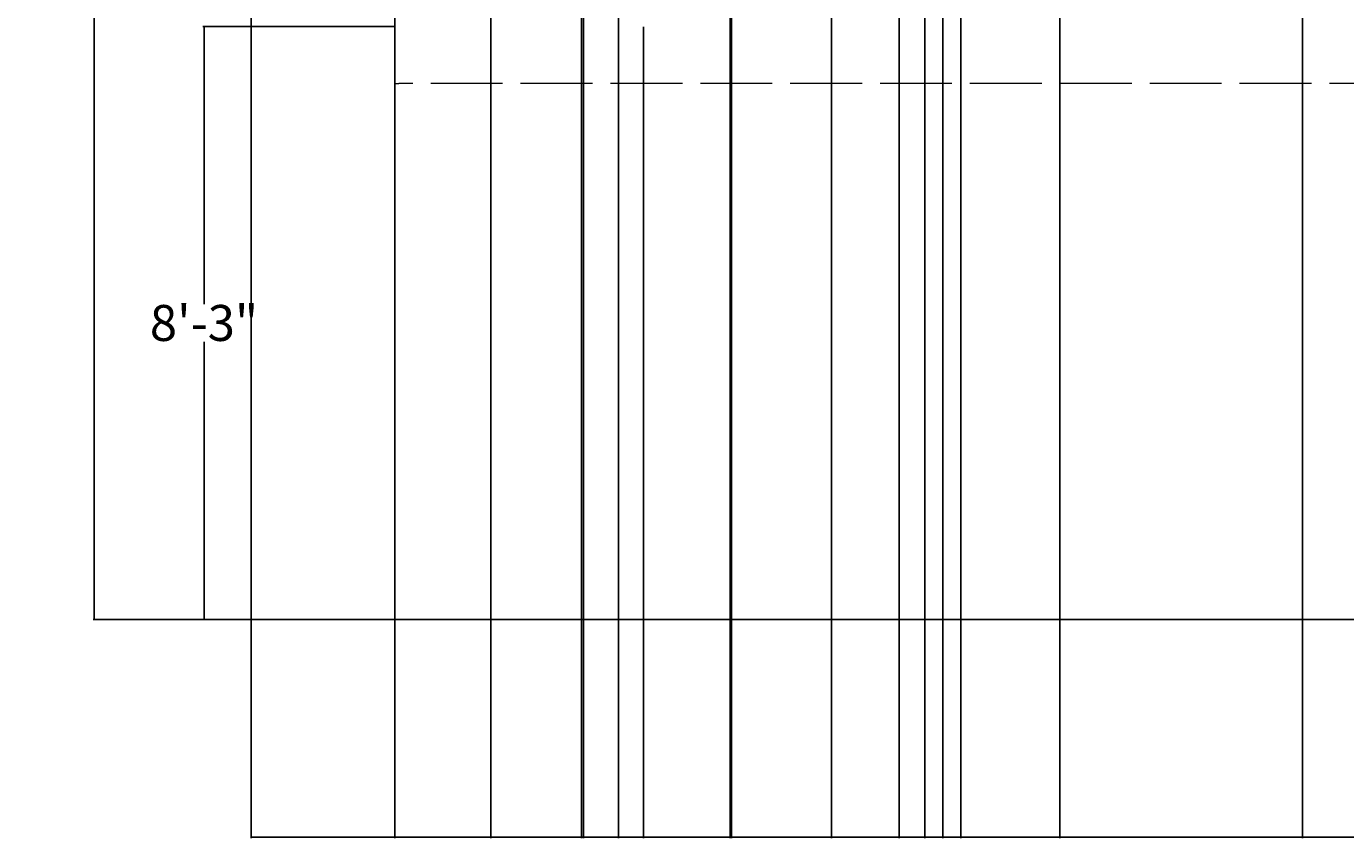
# Model space of a CAD drawing. Units: inches. Extents: x -36 to 401, y -686 to 73.
# Tile 1 of 15: x -36 to 184, y -686 to -550. Entities that reach past the tile are written whole.
import ezdxf

# ---------------------------------------------------------------- set-up
doc = ezdxf.new("R2010")
doc.units = ezdxf.units.IN
doc.header["$MEASUREMENT"] = 0
doc.linetypes.add('ACAD_ISO02W100', pattern=[15, 12, -3])
for name, color, linetype, lineweight in [('A-ANNO-DIMS', 2, 'Continuous', 18), ('A-FLOR-OVHD', 8, 'ACAD_ISO02W100', 18), ('C-PROP', 7, 'Continuous', 25)]:
    doc.layers.add(name, color=color, linetype=linetype, lineweight=lineweight)
doc.styles.get("Standard").update_dxf_attribs({"font": 'arial.ttf'})
doc.dimstyles.get("Standard").update_dxf_attribs({"dimtxt": 0.18, "dimasz": 0.18, "dimexe": 0.18, "dimexo": 0.0625, "dimgap": 0.09, "dimtad": 0, "dimtih": 1, "dimtoh": 1, "dimdec": 0, "dimzin": 0, "dimdsep": 46, "dimlunit": 3, "dimtxsty": 'Standard', "dimcen": 0.09, "dimadec": 0, "dimazin": 0, "dimtfac": 1, "dimtdec": 0, "dimtofl": 0, "dimtmove": 0, "dimatfit": 3, "dimfxl": 1, "dimtolj": 1, "dimtzin": 0, "dimarcsym": 0})

# ---------------------------------------------------------------- blocks, each defined once
blk = doc.blocks.new('*D8')
at = {"layer": 'A-ANNO-DIMS', "color": 0, "lineweight": -2, "transparency": 16777216}
for p, q in [((25.63, 7.79), (-24.68, 7.79)), ((-24.5, 7.61), (-24.5, -317.56)), ((-24.5, -649.03), (-24.5, -323.86)), ((1.63, -649.21), (-24.68, -649.21))]:
    blk.add_line(p, q, dxfattribs=at)
at = {"layer": 'A-ANNO-DIMS', "color": 0, "transparency": 16777216}
for points in [[(-24.53, 7.61), (-24.47, 7.61), (-24.5, 7.79)], [(-24.53, -649.03), (-24.47, -649.03), (-24.5, -649.21)]]:
    blk.add_solid(points, dxfattribs=at)
at = {"layer": 'Defpoints', "color": 0, "transparency": 16777216}
for p in [(25.69, 7.79), (-24.5, -649.21), (1.69, -649.21)]:
    blk.add_point(p, dxfattribs=at)
at = {"layer": 'A-ANNO-DIMS', "color": 0, "transparency": 16777216, "insert": (-24.5, -320.71), "char_height": 6, "attachment_point": 5}
blk.add_mtext('\\A1;54\'-9"', dxfattribs=at)
blk = doc.blocks.new('*D12')
at = {"layer": 'A-ANNO-DIMS', "color": 0, "lineweight": -2, "transparency": 16777216}
for p, q in [((25.63, -550.21), (-6.34, -550.21)), ((-6.16, -550.39), (-6.16, -596.55)), ((-6.16, -649.03), (-6.16, -602.87)), ((25.63, -649.21), (-6.34, -649.21))]:
    blk.add_line(p, q, dxfattribs=at)
at = {"layer": 'A-ANNO-DIMS', "color": 0, "transparency": 16777216}
for points in [[(-6.19, -550.39), (-6.13, -550.39), (-6.16, -550.21)], [(-6.19, -649.03), (-6.13, -649.03), (-6.16, -649.21)]]:
    blk.add_solid(points, dxfattribs=at)
at = {"layer": 'Defpoints', "color": 0, "transparency": 16777216}
for p in [(25.69, -550.21), (-6.16, -649.21), (25.69, -649.21)]:
    blk.add_point(p, dxfattribs=at)
at = {"layer": 'A-ANNO-DIMS', "color": 0, "transparency": 16777216, "insert": (-6.16, -599.71), "char_height": 6, "attachment_point": 5}
blk.add_mtext('\\A1;8\'-3"', dxfattribs=at)
blk = doc.blocks.new('*D64')
at = {"layer": 'A-ANNO-DIMS', "color": 0, "lineweight": -2, "transparency": 16777216}
for p, q in [((1.69, -649.27), (1.69, -685.69)), ((223.02, -649.27), (223.02, -685.69)), ((1.87, -685.51), (111.75, -685.51)), ((222.84, -685.51), (112.95, -685.51))]:
    blk.add_line(p, q, dxfattribs=at)
at = {"layer": 'A-ANNO-DIMS', "color": 0, "transparency": 16777216}
for points in [[(1.87, -685.48), (1.87, -685.54), (1.69, -685.51)], [(222.84, -685.48), (222.84, -685.54), (223.02, -685.51)]]:
    blk.add_solid(points, dxfattribs=at)
at = {"layer": 'Defpoints', "color": 0, "transparency": 16777216}
for p in [(1.69, -649.21), (223.02, -649.21), (223.02, -685.51)]:
    blk.add_point(p, dxfattribs=at)
at = {"layer": 'A-ANNO-DIMS', "color": 0, "transparency": 16777216, "insert": (112.35, -685.51), "char_height": 0.18, "attachment_point": 5}
blk.add_mtext('\\A1;18\'-5 1/2"', dxfattribs=at)
blk = doc.blocks.new('*D65')
at = {"layer": 'A-ANNO-DIMS', "color": 0, "lineweight": -2, "transparency": 16777216}
for p, q in [((67.19, -550.27), (67.19, -685.69)), ((177.19, -550.27), (177.19, -685.69)), ((67.37, -685.51), (121.86, -685.51)), ((177.01, -685.51), (122.52, -685.51))]:
    blk.add_line(p, q, dxfattribs=at)
at = {"layer": 'A-ANNO-DIMS', "color": 0, "transparency": 16777216}
for points in [[(67.37, -685.48), (67.37, -685.54), (67.19, -685.51)], [(177.01, -685.48), (177.01, -685.54), (177.19, -685.51)]]:
    blk.add_solid(points, dxfattribs=at)
at = {"layer": 'Defpoints', "color": 0, "transparency": 16777216}
for p in [(67.19, -550.21), (177.19, -550.21), (177.19, -685.51)]:
    blk.add_point(p, dxfattribs=at)
at = {"layer": 'A-ANNO-DIMS', "color": 0, "transparency": 16777216, "insert": (122.19, -685.51), "char_height": 0.18, "attachment_point": 5}
blk.add_mtext('\\A1;9\'-2"', dxfattribs=at)
blk = doc.blocks.new('*D73')
at = {"layer": 'A-ANNO-DIMS', "color": 0, "lineweight": -2, "transparency": 16777216}
for p, q in [((177.19, -421.27), (177.19, -685.69)), ((253.69, -421.27), (253.69, -685.69)), ((177.37, -685.51), (214.9, -685.51)), ((253.51, -685.51), (215.98, -685.51))]:
    blk.add_line(p, q, dxfattribs=at)
at = {"layer": 'A-ANNO-DIMS', "color": 0, "transparency": 16777216}
for points in [[(177.37, -685.48), (177.37, -685.54), (177.19, -685.51)], [(253.51, -685.48), (253.51, -685.54), (253.69, -685.51)]]:
    blk.add_solid(points, dxfattribs=at)
at = {"layer": 'Defpoints', "color": 0, "transparency": 16777216}
for p in [(177.19, -421.21), (253.69, -421.21), (253.69, -685.51)]:
    blk.add_point(p, dxfattribs=at)
at = {"layer": 'A-ANNO-DIMS', "color": 0, "transparency": 16777216, "insert": (215.44, -685.51), "char_height": 0.18, "attachment_point": 5}
blk.add_mtext('\\A1;6\'-4 1/2"', dxfattribs=at)
blk = doc.blocks.new('*D75')
at = {"layer": 'A-ANNO-DIMS', "color": 0, "lineweight": -2, "transparency": 16777216}
for p, q in [((25.69, -472.27), (25.69, -685.69)), ((57.17, -472.27), (57.17, -685.69)), ((25.87, -685.51), (40.89, -685.51)), ((56.99, -685.51), (41.97, -685.51))]:
    blk.add_line(p, q, dxfattribs=at)
at = {"layer": 'A-ANNO-DIMS', "color": 0, "transparency": 16777216}
for points in [[(25.87, -685.48), (25.87, -685.54), (25.69, -685.51)], [(56.99, -685.48), (56.99, -685.54), (57.17, -685.51)]]:
    blk.add_solid(points, dxfattribs=at)
at = {"layer": 'Defpoints', "color": 0, "transparency": 16777216}
for p in [(25.69, -472.21), (57.17, -472.21), (57.17, -685.51)]:
    blk.add_point(p, dxfattribs=at)
at = {"layer": 'A-ANNO-DIMS', "color": 0, "transparency": 16777216, "insert": (41.43, -685.51), "char_height": 0.18, "attachment_point": 5}
blk.add_mtext('\\A1;2\'-7 1/2"', dxfattribs=at)
blk = doc.blocks.new('*D76')
at = {"layer": 'A-ANNO-DIMS', "color": 0, "lineweight": -2, "transparency": 16777216}
for p, q in [((117.19, -472.27), (117.19, -685.69)), ((136.69, -472.27), (136.69, -685.69)), ((117.37, -685.51), (126.41, -685.51)), ((136.51, -685.51), (127.47, -685.51))]:
    blk.add_line(p, q, dxfattribs=at)
at = {"layer": 'A-ANNO-DIMS', "color": 0, "transparency": 16777216}
for points in [[(117.37, -685.48), (117.37, -685.54), (117.19, -685.51)], [(136.51, -685.48), (136.51, -685.54), (136.69, -685.51)]]:
    blk.add_solid(points, dxfattribs=at)
at = {"layer": 'Defpoints', "color": 0, "transparency": 16777216}
for p in [(117.19, -472.21), (136.69, -472.21), (136.69, -685.51)]:
    blk.add_point(p, dxfattribs=at)
at = {"layer": 'A-ANNO-DIMS', "color": 0, "transparency": 16777216, "insert": (126.94, -685.51), "char_height": 0.18, "attachment_point": 5}
blk.add_mtext('\\A1;1\'-7 1/2"', dxfattribs=at)
blk = doc.blocks.new('*D80')
at = {"layer": 'A-ANNO-DIMS', "color": 0, "lineweight": -2, "transparency": 16777216}
for p, q in [((56.84, -435.52), (56.84, -685.69)), ((120.19, -435.52), (120.19, -685.69)), ((57.02, -685.51), (87.97, -685.51)), ((120.01, -685.51), (89.05, -685.51))]:
    blk.add_line(p, q, dxfattribs=at)
at = {"layer": 'A-ANNO-DIMS', "color": 0, "transparency": 16777216}
for points in [[(57.02, -685.48), (57.02, -685.54), (56.84, -685.51)], [(120.01, -685.48), (120.01, -685.54), (120.19, -685.51)]]:
    blk.add_solid(points, dxfattribs=at)
at = {"layer": 'Defpoints', "color": 0, "transparency": 16777216}
for p in [(56.84, -435.46), (120.19, -435.46), (120.19, -685.51)]:
    blk.add_point(p, dxfattribs=at)
at = {"layer": 'A-ANNO-DIMS', "color": 0, "transparency": 16777216, "insert": (88.51, -685.51), "char_height": 0.18, "attachment_point": 5}
blk.add_mtext('\\A1;5\'-3 1/2"', dxfattribs=at)
blk = doc.blocks.new('*D81')
at = {"layer": 'A-ANNO-DIMS', "color": 0, "lineweight": -2, "transparency": 16777216}
for p, q in [((63, -434.2), (63, -685.69)), ((81.66, -434.2), (81.66, -685.69)), ((63.18, -685.51), (71.8, -685.51)), ((81.48, -685.51), (72.86, -685.51))]:
    blk.add_line(p, q, dxfattribs=at)
at = {"layer": 'A-ANNO-DIMS', "color": 0, "transparency": 16777216}
for points in [[(63.18, -685.48), (63.18, -685.54), (63, -685.51)], [(81.48, -685.48), (81.48, -685.54), (81.66, -685.51)]]:
    blk.add_solid(points, dxfattribs=at)
at = {"layer": 'Defpoints', "color": 0, "transparency": 16777216}
for p in [(63, -434.14), (81.66, -434.14), (81.66, -685.51)]:
    blk.add_point(p, dxfattribs=at)
at = {"layer": 'A-ANNO-DIMS', "color": 0, "transparency": 16777216, "insert": (72.33, -685.51), "char_height": 0.18, "attachment_point": 5}
blk.add_mtext('\\A1;1\'-6 1/2"', dxfattribs=at)
blk = doc.blocks.new('*D83')
at = {"layer": 'A-ANNO-DIMS', "color": 0, "lineweight": -2, "transparency": 16777216}
for p, q in [((56.84, -435.52), (56.84, -685.69)), ((63, -434.2), (63, -685.69)), ((57.02, -685.51), (59.59, -685.51)), ((62.82, -685.51), (60.25, -685.51))]:
    blk.add_line(p, q, dxfattribs=at)
at = {"layer": 'A-ANNO-DIMS', "color": 0, "transparency": 16777216}
for points in [[(57.02, -685.48), (57.02, -685.54), (56.84, -685.51)], [(62.82, -685.48), (62.82, -685.54), (63, -685.51)]]:
    blk.add_solid(points, dxfattribs=at)
at = {"layer": 'Defpoints', "color": 0, "transparency": 16777216}
for p in [(56.84, -435.46), (63, -434.14), (63, -685.51)]:
    blk.add_point(p, dxfattribs=at)
at = {"layer": 'A-ANNO-DIMS', "color": 0, "transparency": 16777216, "insert": (59.92, -685.51), "char_height": 0.18, "attachment_point": 5}
blk.add_mtext('\\A1;0\'-6"', dxfattribs=at)
blk = doc.blocks.new('*D84')
at = {"layer": 'A-ANNO-DIMS', "color": 0, "lineweight": -2, "transparency": 16777216}
for p, q in [((98.57, -433.72), (98.57, -685.69)), ((81.66, -434.2), (81.66, -685.69)), ((81.84, -685.51), (89.79, -685.51)), ((98.39, -685.51), (90.43, -685.51))]:
    blk.add_line(p, q, dxfattribs=at)
at = {"layer": 'A-ANNO-DIMS', "color": 0, "transparency": 16777216}
for points in [[(81.84, -685.48), (81.84, -685.54), (81.66, -685.51)], [(98.39, -685.48), (98.39, -685.54), (98.57, -685.51)]]:
    blk.add_solid(points, dxfattribs=at)
at = {"layer": 'Defpoints', "color": 0, "transparency": 16777216}
for p in [(98.57, -433.66), (81.66, -434.14), (98.57, -685.51)]:
    blk.add_point(p, dxfattribs=at)
at = {"layer": 'A-ANNO-DIMS', "color": 0, "transparency": 16777216, "insert": (90.11, -685.51), "char_height": 0.18, "attachment_point": 5}
blk.add_mtext('\\A1;1\'-5"', dxfattribs=at)
blk = doc.blocks.new('*D85')
at = {"layer": 'A-ANNO-DIMS', "color": 0, "lineweight": -2, "transparency": 16777216}
for p, q in [((114.18, -126.31), (114.18, -685.69)), ((41.7, -137.56), (41.7, -685.69)), ((41.88, -685.51), (77.4, -685.51)), ((114, -685.51), (78.48, -685.51))]:
    blk.add_line(p, q, dxfattribs=at)
at = {"layer": 'A-ANNO-DIMS', "color": 0, "transparency": 16777216}
for points in [[(41.88, -685.48), (41.88, -685.54), (41.7, -685.51)], [(114, -685.48), (114, -685.54), (114.18, -685.51)]]:
    blk.add_solid(points, dxfattribs=at)
at = {"layer": 'Defpoints', "color": 0, "transparency": 16777216}
for p in [(114.18, -126.25), (41.7, -137.5), (114.18, -685.51)]:
    blk.add_point(p, dxfattribs=at)
at = {"layer": 'A-ANNO-DIMS', "color": 0, "transparency": 16777216, "insert": (77.94, -685.51), "char_height": 0.18, "attachment_point": 5}
blk.add_mtext('\\A1;6\'-0 1/2"', dxfattribs=at)
blk = doc.blocks.new('*D89')
at = {"layer": 'A-ANNO-DIMS', "color": 0, "lineweight": -2, "transparency": 16777216}
for p, q in [((81.9, -256.42), (81.9, -685.69)), ((109.9, -256.42), (109.9, -685.69)), ((82.08, -685.51), (95.57, -685.51)), ((109.72, -685.51), (96.23, -685.51))]:
    blk.add_line(p, q, dxfattribs=at)
at = {"layer": 'A-ANNO-DIMS', "color": 0, "transparency": 16777216}
for points in [[(82.08, -685.48), (82.08, -685.54), (81.9, -685.51)], [(109.72, -685.48), (109.72, -685.54), (109.9, -685.51)]]:
    blk.add_solid(points, dxfattribs=at)
at = {"layer": 'Defpoints', "color": 0, "transparency": 16777216}
for p in [(81.9, -256.36), (109.9, -256.36), (109.9, -685.51)]:
    blk.add_point(p, dxfattribs=at)
at = {"layer": 'A-ANNO-DIMS', "color": 0, "transparency": 16777216, "insert": (95.9, -685.51), "char_height": 0.18, "attachment_point": 5}
blk.add_mtext('\\A1;2\'-4"', dxfattribs=at)

msp = doc.modelspace()

# ---------------------------------------------------------------- linework, layer by layer
at = {"layer": 'A-FLOR-OVHD'}
for p, q in [((25.69, -550.21), (25.69, -559.77)), ((25.69, -559.77), (26.38, -559.77)), ((358.69, -559.77), (26.38, -559.77)), ((26.38, -559.77), (26.38, -559.77))]:
    msp.add_line(p, q, dxfattribs=at)
at = {"layer": 'C-PROP'}
for p, q in [((1.69, 31.79), (1.69, -649.21)), ((1.69, -649.21), (223.02, -649.21))]:
    msp.add_line(p, q, dxfattribs=at)

# ---------------------------------------------------------------- dimensions: what is measured, and where the dimension line sits
at = {"layer": 'A-ANNO-DIMS'}
for base, p1, p2, picture, middle in [((-24.5, -649.21), (25.69, 7.79), (1.69, -649.21), '*D8', (-24.5, -320.71)), ((-6.16, -649.21), (25.69, -550.21), (25.69, -649.21), '*D12', (-6.16, -599.71))]:
    dim = msp.add_linear_dim(base=base, p1=p1, p2=p2, angle=90, dimstyle='Standard', override={"dimtxt": 6, "dimclrd": 0, "dimclre": 0, "dimclrt": 0}, dxfattribs=at)
    dim.commit()
    dim.dimension.update_dxf_attribs({"geometry": picture, "text_midpoint": middle})
for base, p1, p2, picture, middle in [((114.18, -685.51), (41.7, -137.5), (114.18, -126.25), '*D85', (77.94, -685.51)), ((109.9, -685.51), (81.9, -256.36), (109.9, -256.36), '*D89', (95.9, -685.51)), ((253.69, -685.51), (177.19, -421.21), (253.69, -421.21), '*D73', (215.44, -685.51)), ((98.57, -685.51), (81.66, -434.14), (98.57, -433.66), '*D84', (90.11, -685.51)), ((63, -685.51), (56.84, -435.46), (63, -434.14), '*D83', (59.92, -685.51)), ((120.1884, -685.5099), (56.8374, -435.458), (120.1884, -435.458), '*D80', (88.5129, -685.5099)), ((81.66, -685.51), (63, -434.14), (81.66, -434.14), '*D81', (72.33, -685.51)), ((57.17, -685.51), (25.69, -472.21), (57.17, -472.21), '*D75', (41.43, -685.51)), ((136.69, -685.51), (117.19, -472.21), (136.69, -472.21), '*D76', (126.94, -685.51)), ((177.19, -685.51), (67.19, -550.21), (177.19, -550.21), '*D65', (122.19, -685.51)), ((223.02, -685.51), (1.69, -649.21), (223.02, -649.21), '*D64', (112.35, -685.51))]:
    dim = msp.add_linear_dim(base=base, p1=p1, p2=p2, dimstyle='Standard', override={"dimdec": 1, "dimlfac": 1, "dimrnd": 0, "dimzin": 1, "dimdsep": 46, "dimlunit": 4, "dimfrac": 2}, dxfattribs=at)
    dim.commit()
    dim.dimension.update_dxf_attribs({"geometry": picture, "text_midpoint": middle})

doc.saveas('drawing.dxf')
